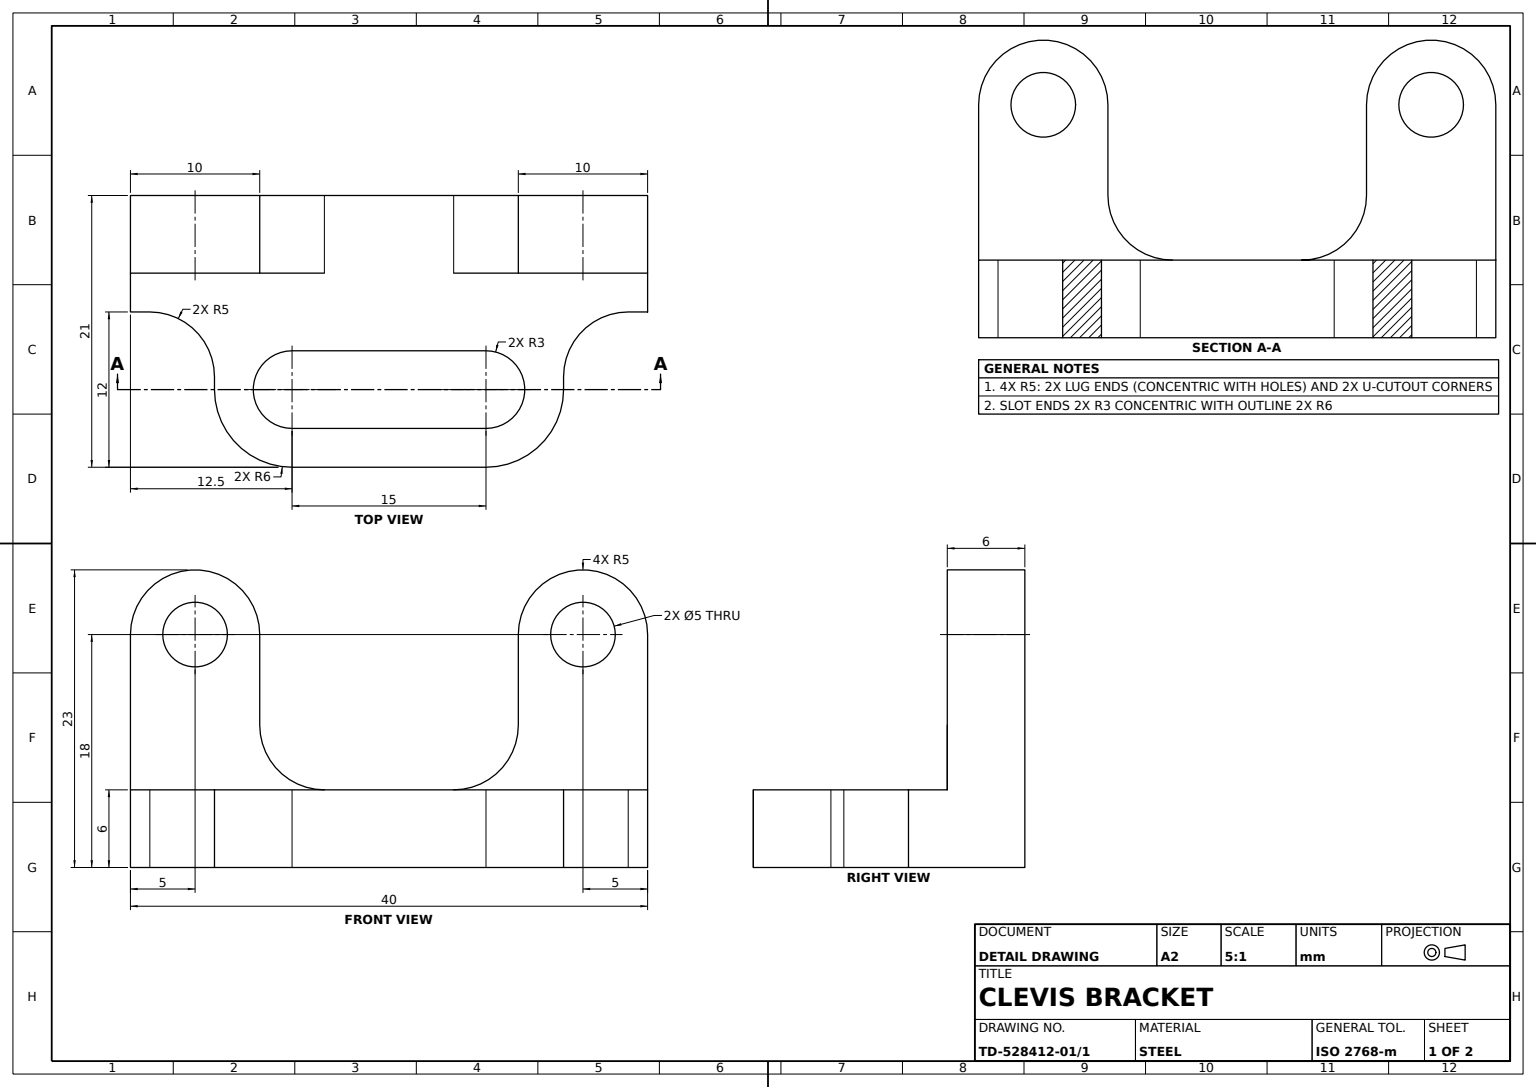
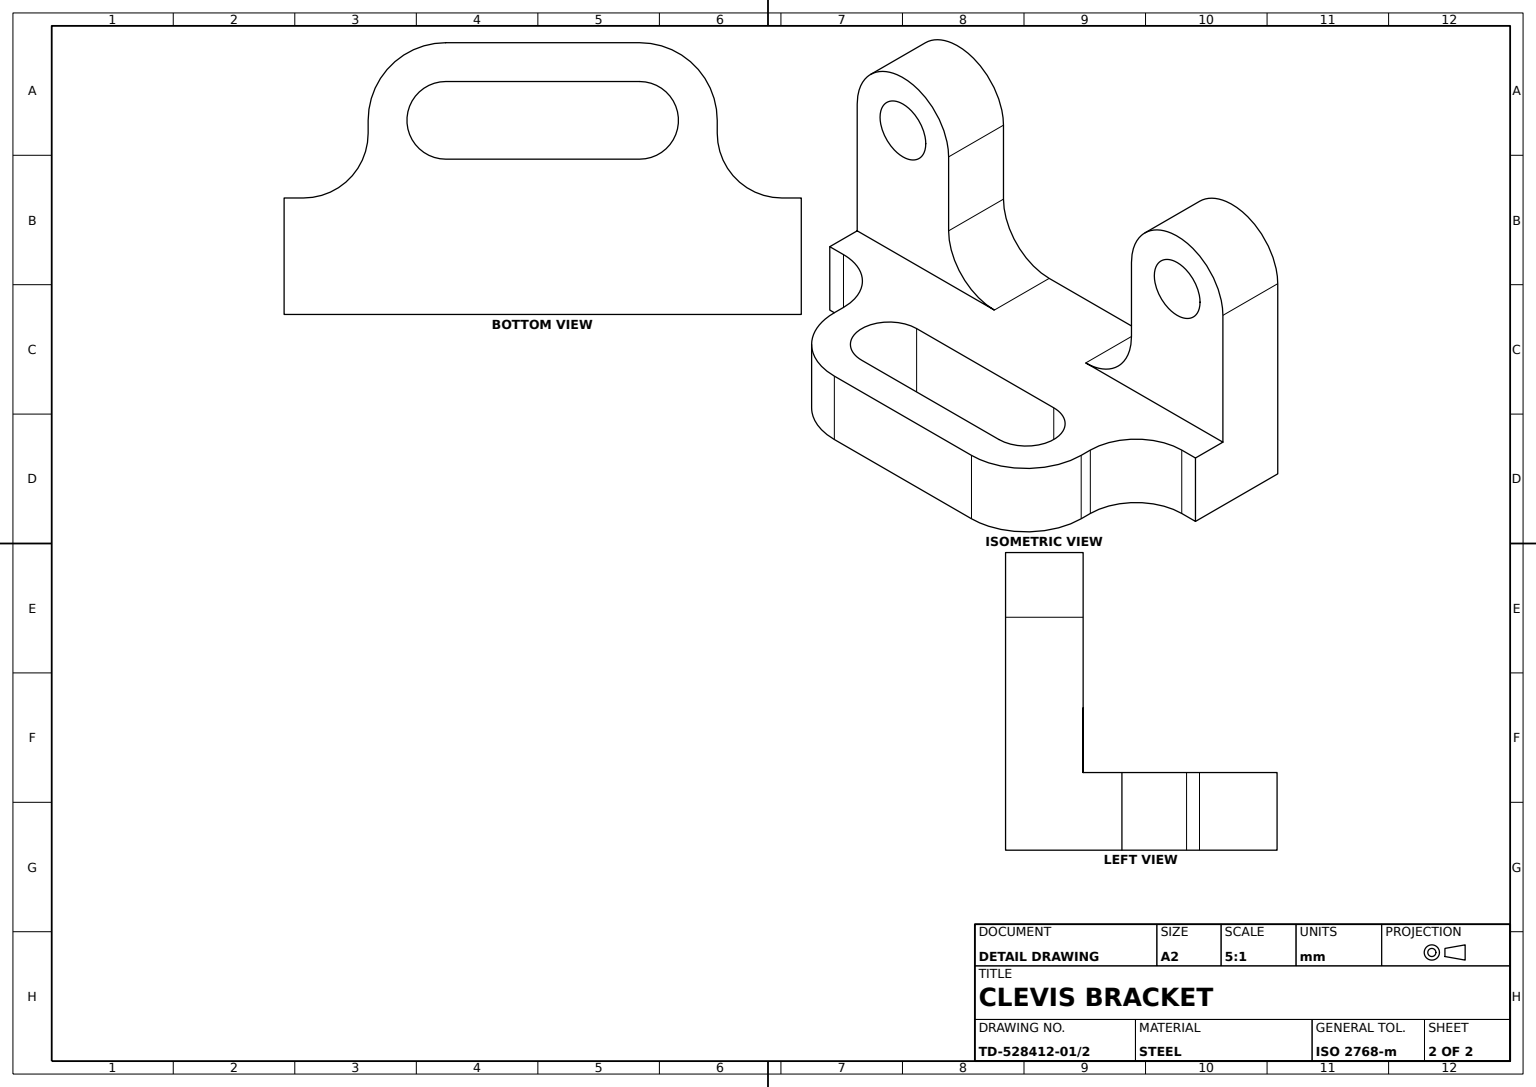
SolidWorks part; units mm, degrees
material "Plain Carbon Steel"
ref_plane "Front Plane" through (0, 0, 0) normal (0, 0, 1) x (1, 0, 0)
ref_plane "Top Plane" through (0, 0, 0) normal (0, 1, 0) x (1, 0, 0)
ref_plane "Right Plane" through (0, 0, 0) normal (1, 0, 0) x (0, 0, -1)
sketch "Base Plate Profile" plane through (0, 0, 0) normal (0, 1, 0) x (1, 0, 0)
  line L0 (-20, 0) -> (20, 0)
  line L1 (-12.65, 0) -> (12.65, 0) construction
  line L2 (-20, 0) -> (-20, -6)
  line L3 (18.5, -6) -> (20, -6)
  line L4 (20, -6) -> (20, 0)
  line L5 (0, -12) -> (0, -18)
  line L6 (-7.5, -18) -> (7.5, -18)
  line L7 (-13.5, -12) -> (-13.5, -11)
  line L8 (13.5, -12) -> (13.5, -11)
  line L9 (-20, -6) -> (-18.5, -6)
  line L10 (0, -18) -> (0, -12)
  line L11 (-7.5, -12) -> (7.5, -12) construction
  line L12 (-7.5, -9) -> (7.5, -9)
  line L13 (-7.5, -15) -> (7.5, -15)
  arc A0 (13.5, -11) -> (18.5, -6) centre (18.5, -11) cw
  arc A1 (-13.5, -11) -> (-18.5, -6) centre (-18.5, -11) ccw
  arc A2 (13.5, -12) -> (7.5, -18) centre (7.5, -12) cw
  arc A3 (-7.5, -18) -> (-13.5, -12) centre (-7.5, -12) cw
  arc A4 (-7.5, -9) -> (-7.5, -15) centre (-7.5, -12) ccw
  arc A5 (7.5, -15) -> (7.5, -9) centre (7.5, -12) ccw
  point P6 (0, 0)
  point P14 (0, -18)
  point P20 (-13.5, -6)
  point P27 (0, -12)
  dimension "D2" = 5
  dimension "D4" = 5
  dimension "D5" = 6
  dimension "D7" = 3
  dimension "D1" = 40
  dimension "D3" = 6
  dimension "D6" = 15
  dimension "D8" = 1
  dimension "D9" = 6
extrude "Base Plate" add sketch "Base Plate Profile" along normal mid plane 6
sketch "Clevis Lugs Profile" plane through (0, 0, 0) normal (0, 0, -1) x (-1, 0, 0)
  line L0 (-20, -3) -> (-20, 15)
  line L1 (20, -3) -> (20, 15)
  line L2 (-10, 15) -> (-10, 8)
  line L3 (20, 3) -> (-20, 3) construction
  line L4 (10, 15) -> (10, 8)
  line L5 (5, 3) -> (-5, 3)
  line L6 (-20, -3) -> (20, -3)
  line L7 (-5, 3) -> (20, 3)
  line L8 (-20, 3) -> (-20, -3)
  line L10 (20, 3) -> (20, -3)
  circle A0 centre (-15, 15) radius 2.5
  circle A1 centre (15, 15) radius 2.5
  circle A2 centre (-15, 15) radius 5
  circle A3 centre (15, 15) radius 5
  arc A4 (5, 3) -> (10, 8) centre (5, 8) ccw
  arc A5 (-10, 8) -> (-5, 3) centre (-5, 8) ccw
  line M6 (-20, -3) -> (20, -3)
  line M7 (20, -3) -> (20, 3)
  line M8 (20, 3) -> (-20, 3)
  line M9 (-20, 3) -> (-20, -3)
  dimension "D3" = 5
  dimension "D4" = 5
  dimension "D7" = 5
  dimension "D1" = 18
  dimension "D2" = 18
  dimension "D5" = 5
  dimension "D6" = 5
  dimension "D8" = 10
  dimension "D9" = 10
extrude "Clevis Lugs" add sketch "Clevis Lugs Profile" along normal mid plane 6 contours M9 M6 M7 M8 | A5 L2 A2 L0 M8 | A4 L1 A3 L4 M8 | A3 A1 | A2 A0
